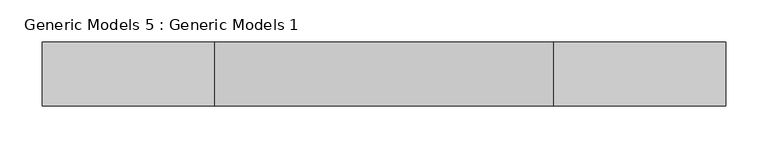
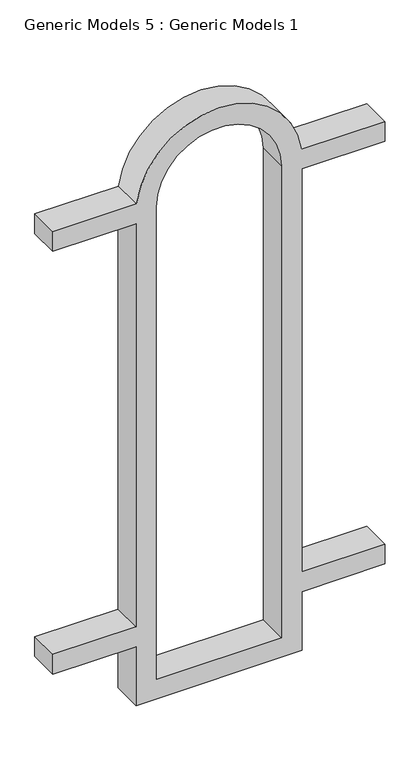
"""IFC4 building model written with IfcOpenShell, lengths in millimetres: proxy geometry, Generic Models 5 : Generic Models 1."""

from ifc_helpers import new_model, si_unit, point, frame, frame_2d, origin, place, context, project, spatial, polyline, circle_curve, trimmed, segment, composite_curve, outline, extrude, source, transform, mapped, element, save


def generic_models_5_generic_models_1_f7cfe2cb(model_context):
    return source(origin(), model_context, "Body", "SweptSolid", [
        extrude(outline(composite_curve([segment(polyline([(1905.0, -7057.8887575), (1905.0, -7262.6825076), (1854.2, -7262.6825076), (1854.2, -7059.4825076), (812.8, -7059.4825076), (812.8, -7262.6825076), (762.0, -7262.6825076), (762.0, -7059.4825076), (609.6, -7059.4825076), (609.6, -6653.0825076), (762.0, -6653.0825076), (762.0, -6449.8825076), (812.8, -6449.8825076), (812.8, -6653.0825076), (1854.2, -6653.0825076), (1854.2, -6449.8825076), (1905.0, -6449.8825076), (1905.0, -6654.6762577)]), True, "CONTINUOUS"), segment(trimmed(circle_curve(frame_2d((1879.6, -6856.2825076)), 203.2), [point((1905.0, -6654.6762577))], [point((1905.0, -7057.8887575))], False, "CARTESIAN"), True, "CONTINUOUS")], self_intersect=False), holes=[composite_curve([segment(trimmed(circle_curve(frame_2d((1879.6, -6856.2825076)), 152.4), [point((1879.6, -7008.6825076))], [point((1879.6, -6703.8825076))], True, "CARTESIAN"), True, "CONTINUOUS"), segment(polyline([(1879.6, -6703.8825076), (660.4, -6703.8825076), (660.4, -7008.6825076), (1879.6, -7008.6825076)]), True, "CONTINUOUS")], self_intersect=False)]), frame((0.0, -4810.2608295, 0.0), z_axis=(0.0, 1.0, 0.0), x_axis=(0.0, 0.0, 1.0)), (0.0, 0.0, 1.0), 76.2),
    ])


if __name__ == "__main__":
    model = new_model("IFC4")
    model_context = context("Model", 3, world=origin())
    ifc_project = project(units=[si_unit("LENGTHUNIT", "METRE", prefix="MILLI")], contexts=[model_context])
    site = spatial("IfcSite", under=ifc_project)
    building = spatial("IfcBuilding", under=site)
    placement = place(None, origin())
    generic_models_5_generic_models_1_shape = generic_models_5_generic_models_1_f7cfe2cb(model_context)
    element("IfcBuildingElementProxy", 1, Name="Generic Models 5 : Generic Models 1", ObjectType="Generic Models 5 : Generic Models 1", at=placement, inside=building, context=model_context, shape_type="MappedRepresentation", body=[
        mapped(generic_models_5_generic_models_1_shape, transform((0.0, 0.0, 0.0), x_axis=(1.0, 0.0, 0.0), y_axis=(0.0, 1.0, 0.0), z_axis=(0.0, 0.0, 1.0))),
    ])
    save(model, "model.ifc")

# Revit data of these elements
# Element 1 (IfcBuildingElementProxy, "Generic Models 5 : Generic Models 1")
#   Materials on its faces: "Aluminum"
# Materials
#   "Aluminum": class "Metal", colour RGB 244 245 246, transparency 0, Description = "Aluminum 6061", Cost = 0
